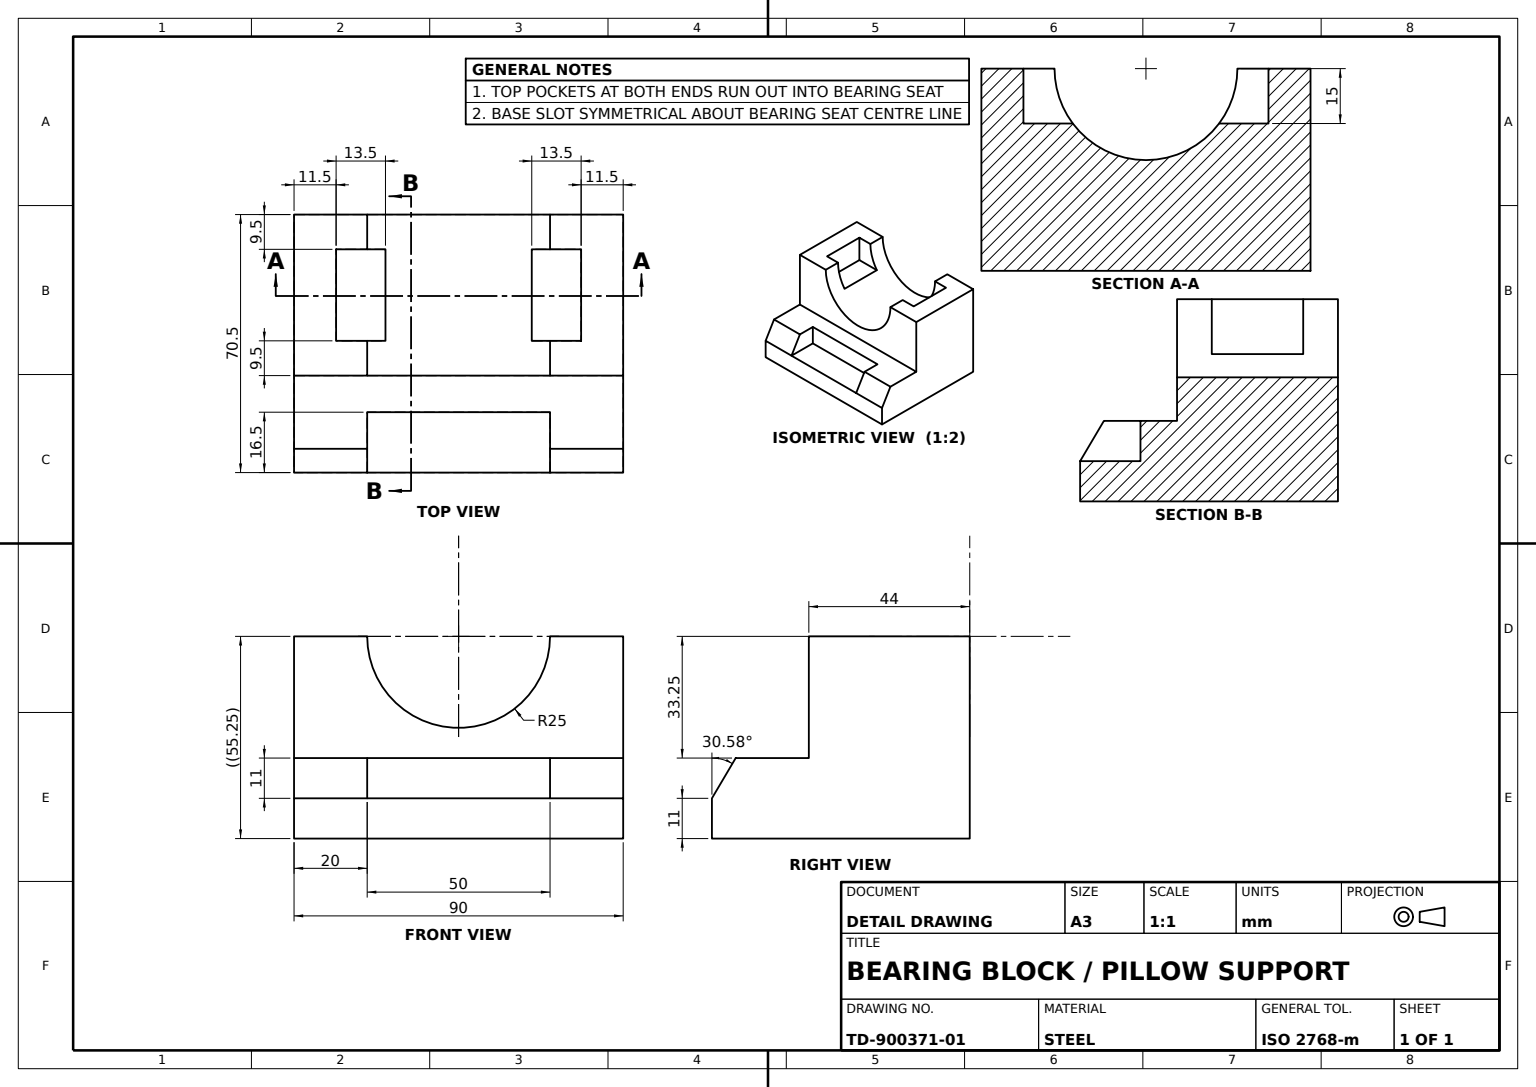
from build123d import *

# Parameters (mm, degrees)
BRACKET_PROFILE_SKETCH_W = 44
BRACKET_PROFILE_SKETCH_H = 55.25
BRACKET_BODY_DEPTH       = 45
BEARING_SEAT_R25_DEPTH   = 45
BASE_SLOT_SKETCH_W       = 16.5
BASE_SLOT_SKETCH_H       = 50
BASE_MOUNTING_SLOT_DEPTH = 11
TOP_RECESSES_DEPTH       = 15


with BuildPart() as part:
    # Bracket Profile Sketch → Bracket Body (new, symmetric)
    with BuildSketch(Plane.XY):
        with Locations((22, 27.625)):
            Rectangle(BRACKET_PROFILE_SKETCH_W, BRACKET_PROFILE_SKETCH_H)
        Polygon((44, 22), (44, 0), (70.5, 0), (70.5, 11), (64, 22), align=None)
    extrude(amount=BRACKET_BODY_DEPTH, both=True)

    # Bearing Seat Sketch → Bearing Seat R25 (cut)
    with BuildSketch(Plane(origin=(44, 0, 0), x_dir=(0, 0, -1), z_dir=(1, 0, 0))):
        with BuildLine():
            Line((-25, 55.25), (25, 55.25))
            ThreePointArc((25, 55.25), (0, 30.25), (-25, 55.25))
        make_face()
    extrude(amount=-BEARING_SEAT_R25_DEPTH, mode=Mode.SUBTRACT)

    # Base Slot Sketch → Base Mounting Slot (cut)
    with BuildSketch(Plane(origin=(0, 22, 0), x_dir=(1, 0, 0), z_dir=(0, 1, 0))):
        with Locations((62.25, 0)):
            Rectangle(BASE_SLOT_SKETCH_W, BASE_SLOT_SKETCH_H)
    extrude(amount=-BASE_MOUNTING_SLOT_DEPTH, mode=Mode.SUBTRACT)

    # Top Recess Sketch → Top Recesses (cut)
    with BuildSketch(Plane(origin=(0, 55.25, 0), x_dir=(1, 0, 0), z_dir=(0, 1, 0))):
        Polygon((9.5, -33.5), (22, -33.5), (34.5, -33.5), (34.5, -18.5), (9.5, -18.5), align=None)
        Polygon((22, 33.5), (34.5, 33.5), (34.5, 18.5), (9.5, 18.5), (9.5, 33.5), align=None)
    extrude(amount=-TOP_RECESSES_DEPTH, mode=Mode.SUBTRACT)


solid = part.part
